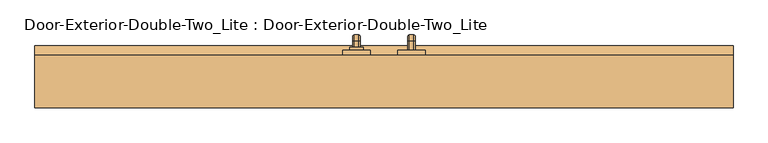
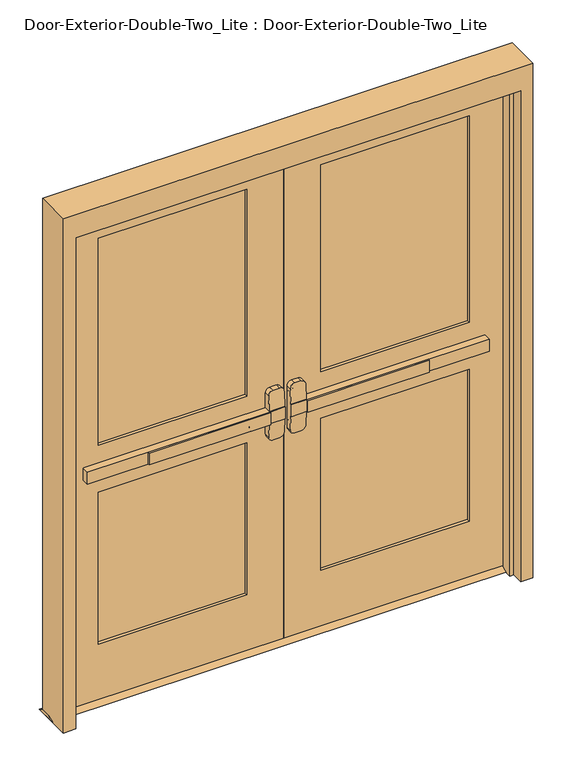
"""IFC4 building model written with IfcOpenShell, lengths in millimetres: door geometry, Door-Exterior-Double-Two_Lite : Door-Exterior-Double-Two_Lite."""

from ifc_helpers import new_model, si_unit, point, frame, frame_2d, origin, place, context, project, spatial, polyline, circle_curve, ellipse_curve, trimmed, segment, composite_curve, outline, extrude, faceted_brep, source, transform, mapped, element, save
from ifc_brep_helpers import plane_surface, cylinder_surface, revolved_surface, advanced_brep


def door_exterior_double_two_lite_door_exterior_double_two_lite_aa7d30b3(model_context):
    return source(origin(), model_context, "Body", "SolidModel", [
        extrude(outline(polyline([(-575.7333333, 48.4), (-575.7333333, 54.75), (-76.2, 54.75), (-76.2, 48.4), (-575.7333333, 48.4)])), frame((0.0, 0.0, 990.6), z_axis=(0.0, 0.0, 1.0), x_axis=(1.0, 0.0, 0.0)), (0.0, 0.0, 1.0), 50.8),
        advanced_brep(
        [(-12.7, 54.75, 1041.4), (-76.2, 54.75, 1041.4), (-825.5, 54.75, 1041.4), (-825.5, 54.75, 990.6), (-76.2, 54.75, 990.6), (-12.7, 54.75, 990.6), (-825.5, 86.5, 1041.4), (-76.2, 86.5, 1041.4), (-76.2, 86.5, 1104.9), (-57.15, 86.5, 1123.95), (-31.75, 86.5, 1123.95), (-12.7, 86.5, 1104.9), (-12.7, 86.5, 927.1), (-31.75, 86.5, 908.05), (-57.15, 86.5, 908.05), (-76.2, 86.5, 927.1), (-76.2, 86.5, 990.6), (-825.5, 86.5, 990.6), (-12.7, 57.9252467, 1041.4), (-76.2, 57.9252467, 1041.4), (-12.7, 57.9252467, 990.6), (-12.7, 62.9354269, 927.1), (-12.7, 62.9354269, 1104.9), (-76.2, 57.9252467, 990.6), (-76.2, 62.9354269, 1104.9), (-76.2, 62.9354269, 927.1), (-57.15, 64.438481, 1123.95), (-31.75, 64.438481, 1123.95), (-31.75, 64.438481, 908.05), (-57.15, 64.438481, 908.05)],
        [
            (0, 1),
            (1, 2),
            (2, 3),
            (3, 4),
            (4, 5),
            (5, 0),
            (6, 7),
            (7, 8),
            (8, 9, circle_curve(frame((-57.15, 86.5, 1104.9), z_axis=(0.0, 1.0, 0.0), x_axis=(-1.0, 0.0, 0.0)), 19.05)),
            (9, 10),
            (10, 11, circle_curve(frame((-31.75, 86.5, 1104.9), z_axis=(0.0, 1.0, 0.0), x_axis=(-1.0, 0.0, 0.0)), 19.05)),
            (11, 12),
            (12, 13, circle_curve(frame((-31.75, 86.5, 927.1), z_axis=(0.0, 1.0, 0.0), x_axis=(-1.0, 0.0, 0.0)), 19.05)),
            (13, 14),
            (14, 15, circle_curve(frame((-57.15, 86.5, 927.1), z_axis=(0.0, 1.0, 0.0), x_axis=(-1.0, 0.0, 0.0)), 19.05)),
            (15, 16),
            (16, 17),
            (17, 6),
            (0, 18),
            (18, 19),
            (19, 7),
            (6, 2),
            (5, 20),
            (20, 21),
            (21, 12),
            (11, 22),
            (22, 18),
            (16, 23),
            (23, 20),
            (3, 17),
            (19, 24),
            (24, 8),
            (15, 25),
            (25, 23),
            (9, 26),
            (26, 27),
            (27, 10),
            (13, 28),
            (28, 29),
            (29, 14),
            (29, 25, ellipse_curve(frame((-57.15, 62.9354269, 927.1), z_axis=(0.0, 0.9969018152893365, 0.07865602756830282), x_axis=(0.0, -0.07865602756830208, 0.9969018152893365)), 19.1092038, 19.05)),
            (24, 26, ellipse_curve(frame((-57.15, 62.9354269, 1104.9), z_axis=(0.0, 0.9969018152893376, -0.07865602756828934), x_axis=(0.0, -0.078656027568288, -0.9969018152893377)), 19.1092038, 19.05)),
            (27, 22, ellipse_curve(frame((-31.75, 62.9354269, 1104.9), z_axis=(0.0, 0.9969018152893376, -0.07865602756828934), x_axis=(0.0, -0.078656027568288, -0.9969018152893377)), 19.1092038, 19.05)),
            (21, 28, ellipse_curve(frame((-31.75, 62.9354269, 927.1), z_axis=(0.0, 0.9969018152893365, 0.07865602756830282), x_axis=(0.0, -0.07865602756830208, 0.9969018152893365)), 19.1092038, 19.05)),
        ],
        [
            plane_surface(frame((-12.7, 54.75, 1041.4), z_axis=(0.0, -1.0, 0.0), x_axis=(1.0, 0.0, 0.0))),
            plane_surface(frame((-12.7, 86.5, 1041.4), z_axis=(0.0, 1.0, 0.0), x_axis=(-1.0, 0.0, 0.0))),
            plane_surface(frame((-825.5, 54.75, 1041.4), z_axis=(0.0, 0.0, 1.0), x_axis=(0.0, 1.0, 0.0))),
            plane_surface(frame((-12.7, 54.75, 1041.4), z_axis=(1.0, 0.0, 0.0), x_axis=(0.0, 1.0, 0.0))),
            plane_surface(frame((-12.7, 54.75, 990.6), z_axis=(0.0, 0.0, -1.0), x_axis=(0.0, 1.0, 0.0))),
            plane_surface(frame((-825.5, 54.75, 990.6), z_axis=(-1.0, 0.0, 0.0), x_axis=(0.0, 1.0, 0.0))),
            plane_surface(frame((-76.2, 57.9252467, 927.1), z_axis=(-1.0, 0.0, 0.0), x_axis=(0.0, 1.0, 0.0))),
            plane_surface(frame((-57.15, 57.9252467, 1123.95), z_axis=(0.0, 0.0, 1.0), x_axis=(0.0, 1.0, 0.0))),
            plane_surface(frame((-31.75, 57.9252467, 908.05), z_axis=(0.0, 0.0, -1.0), x_axis=(0.0, 1.0, 0.0))),
            cylinder_surface(frame((-57.15, 86.5, 927.1), z_axis=(0.0, -1.0, 0.0), x_axis=(-1.0, 0.0, 0.0)), 19.05),
            cylinder_surface(frame((-57.15, 86.5, 1104.9), z_axis=(0.0, -1.0, 0.0), x_axis=(-1.0, 0.0, 0.0)), 19.05),
            cylinder_surface(frame((-31.75, 86.5, 1104.9), z_axis=(0.0, -1.0, 0.0), x_axis=(-1.0, 0.0, 0.0)), 19.05),
            cylinder_surface(frame((-31.75, 86.5, 927.1), z_axis=(0.0, -1.0, 0.0), x_axis=(-1.0, 0.0, 0.0)), 19.05),
            plane_surface(frame((-76.2, 57.9252467, 1041.4), z_axis=(0.0, -0.9969018152893376, 0.07865602756828934), x_axis=(1.0, 0.0, 0.0))),
            plane_surface(frame((-76.2, 64.438481, 908.05), z_axis=(0.0, -0.9969018152893365, -0.07865602756830282), x_axis=(1.0, 0.0, 0.0))),
        ],
        [
            (0, [[1, 2, 3, 4, 5, 6]]),
            (1, [[7, 8, 9, 10, 11, 12, 13, 14, 15, 16, 17, 18]]),
            (2, [[-2, -1, 19, 20, 21, -7, 22]]),
            (3, [[23, 24, 25, -12, 26, 27, -19, -6]]),
            (4, [[-17, 28, 29, -23, -5, -4, 30]]),
            (5, [[-22, -18, -30, -3]]),
            (6, [[-21, 31, 32, -8]]),
            (6, [[33, 34, -28, -16]]),
            (7, [[35, 36, 37, -10]]),
            (8, [[38, 39, 40, -14]]),
            (9, [[-40, 41, -33, -15]]),
            (10, [[-32, 42, -35, -9]]),
            (11, [[-37, 43, -26, -11]]),
            (12, [[-25, 44, -38, -13]]),
            (13, [[-27, -43, -36, -42, -31, -20]]),
            (14, [[-29, -34, -41, -39, -44, -24]]),
        ],
    ),
        extrude(outline(polyline([(130.95, 12.7), (156.35, 0.0), (61.1, 0.0), (86.5, 12.7), (130.95, 12.7)])), frame((-965.2, 0.0, 0.0), z_axis=(1.0, 0.0, 0.0), x_axis=(0.0, 1.0, 0.0)), (0.0, 0.0, 1.0), 1930.4),
        extrude(outline(polyline([(575.7333333, 48.4), (76.2, 48.4), (76.2, 54.75), (575.7333333, 54.75), (575.7333333, 48.4)])), frame((0.0, 0.0, 990.6), z_axis=(0.0, 0.0, 1.0), x_axis=(1.0, 0.0, 0.0)), (0.0, 0.0, 1.0), 50.8),
        advanced_brep(
        [(12.7, 54.75, 1041.4), (12.7, 54.75, 990.6), (76.2, 54.75, 990.6), (825.5, 54.75, 990.6), (825.5, 54.75, 1041.4), (76.2, 54.75, 1041.4), (825.5, 86.5, 1041.4), (825.5, 86.5, 990.6), (76.2, 86.5, 990.6), (76.2, 86.5, 927.1), (57.15, 86.5, 908.05), (31.75, 86.5, 908.05), (12.7, 86.5, 927.1), (12.7, 86.5, 1104.9), (31.75, 86.5, 1123.95), (57.15, 86.5, 1123.95), (76.2, 86.5, 1104.9), (76.2, 86.5, 1041.4), (76.2, 57.9252467, 1041.4), (12.7, 57.9252467, 1041.4), (12.7, 62.9354269, 1104.9), (12.7, 62.9354269, 927.1), (12.7, 57.9252467, 990.6), (76.2, 57.9252467, 990.6), (76.2, 62.9354269, 927.1), (76.2, 62.9354269, 1104.9), (31.75, 64.438481, 1123.95), (57.15, 64.438481, 1123.95), (57.15, 64.438481, 908.05), (31.75, 64.438481, 908.05)],
        [
            (0, 1),
            (1, 2),
            (2, 3),
            (3, 4),
            (4, 5),
            (5, 0),
            (6, 7),
            (7, 8),
            (8, 9),
            (9, 10, circle_curve(frame((57.15, 86.5, 927.1), z_axis=(0.0, 1.0, 0.0), x_axis=(1.0, 0.0, 0.0)), 19.05)),
            (10, 11),
            (11, 12, circle_curve(frame((31.75, 86.5, 927.1), z_axis=(0.0, 1.0, 0.0), x_axis=(1.0, 0.0, 0.0)), 19.05)),
            (12, 13),
            (13, 14, circle_curve(frame((31.75, 86.5, 1104.9), z_axis=(0.0, 1.0, 0.0), x_axis=(1.0, 0.0, 0.0)), 19.05)),
            (14, 15),
            (15, 16, circle_curve(frame((57.15, 86.5, 1104.9), z_axis=(0.0, 1.0, 0.0), x_axis=(1.0, 0.0, 0.0)), 19.05)),
            (16, 17),
            (17, 6),
            (4, 6),
            (17, 18),
            (18, 19),
            (19, 0),
            (19, 20),
            (20, 13),
            (12, 21),
            (21, 22),
            (22, 1),
            (7, 3),
            (22, 23),
            (23, 8),
            (23, 24),
            (24, 9),
            (16, 25),
            (25, 18),
            (14, 26),
            (26, 27),
            (27, 15),
            (10, 28),
            (28, 29),
            (29, 11),
            (24, 28, ellipse_curve(frame((57.15, 62.9354269, 927.1), z_axis=(0.0, 0.9969018152893365, 0.07865602756830282), x_axis=(0.0, -0.07865602756830208, 0.9969018152893365)), 19.1092038, 19.05)),
            (27, 25, ellipse_curve(frame((57.15, 62.9354269, 1104.9), z_axis=(0.0, 0.9969018152893376, -0.07865602756828934), x_axis=(0.0, -0.078656027568288, -0.9969018152893377)), 19.1092038, 19.05)),
            (20, 26, ellipse_curve(frame((31.75, 62.9354269, 1104.9), z_axis=(0.0, 0.9969018152893376, -0.07865602756828934), x_axis=(0.0, -0.078656027568288, -0.9969018152893377)), 19.1092038, 19.05)),
            (29, 21, ellipse_curve(frame((31.75, 62.9354269, 927.1), z_axis=(0.0, 0.9969018152893365, 0.07865602756830282), x_axis=(0.0, -0.07865602756830208, 0.9969018152893365)), 19.1092038, 19.05)),
        ],
        [
            plane_surface(frame((12.7, 54.75, 1041.4), z_axis=(0.0, -1.0, 0.0), x_axis=(-1.0, 0.0, 0.0))),
            plane_surface(frame((12.7, 86.5, 1041.4), z_axis=(0.0, 1.0, 0.0), x_axis=(1.0, 0.0, 0.0))),
            plane_surface(frame((825.5, 54.75, 1041.4), z_axis=(0.0, 0.0, 1.0), x_axis=(0.0, 1.0, 0.0))),
            plane_surface(frame((12.7, 54.75, 1041.4), z_axis=(-1.0, 0.0, 0.0), x_axis=(0.0, 1.0, 0.0))),
            plane_surface(frame((12.7, 54.75, 990.6), z_axis=(0.0, 0.0, -1.0), x_axis=(0.0, 1.0, 0.0))),
            plane_surface(frame((825.5, 54.75, 990.6), z_axis=(1.0, 0.0, 0.0), x_axis=(0.0, 1.0, 0.0))),
            plane_surface(frame((76.2, 57.9252467, 927.1), z_axis=(1.0, 0.0, 0.0), x_axis=(0.0, 1.0, 0.0))),
            plane_surface(frame((57.15, 57.9252467, 1123.95), z_axis=(0.0, 0.0, 1.0), x_axis=(0.0, 1.0, 0.0))),
            plane_surface(frame((31.75, 57.9252467, 908.05), z_axis=(0.0, 0.0, -1.0), x_axis=(0.0, 1.0, 0.0))),
            cylinder_surface(frame((57.15, 86.5, 927.1), z_axis=(0.0, -1.0, 0.0), x_axis=(1.0, 0.0, 0.0)), 19.05),
            cylinder_surface(frame((57.15, 86.5, 1104.9), z_axis=(0.0, -1.0, 0.0), x_axis=(1.0, 0.0, 0.0)), 19.05),
            cylinder_surface(frame((31.75, 86.5, 1104.9), z_axis=(0.0, -1.0, 0.0), x_axis=(1.0, 0.0, 0.0)), 19.05),
            cylinder_surface(frame((31.75, 86.5, 927.1), z_axis=(0.0, -1.0, 0.0), x_axis=(1.0, 0.0, 0.0)), 19.05),
            plane_surface(frame((76.2, 57.9252467, 1041.4), z_axis=(0.0, -0.9969018152893376, 0.07865602756828934), x_axis=(-1.0, 0.0, 0.0))),
            plane_surface(frame((76.2, 64.438481, 908.05), z_axis=(0.0, -0.9969018152893365, -0.07865602756830282), x_axis=(-1.0, 0.0, 0.0))),
        ],
        [
            (0, [[1, 2, 3, 4, 5, 6]]),
            (1, [[7, 8, 9, 10, 11, 12, 13, 14, 15, 16, 17, 18]]),
            (2, [[19, -18, 20, 21, 22, -6, -5]]),
            (3, [[-1, -22, 23, 24, -13, 25, 26, 27]]),
            (4, [[28, -3, -2, -27, 29, 30, -8]]),
            (5, [[-4, -28, -7, -19]]),
            (6, [[-9, -30, 31, 32]]),
            (6, [[-17, 33, 34, -20]]),
            (7, [[-15, 35, 36, 37]]),
            (8, [[-11, 38, 39, 40]]),
            (9, [[-10, -32, 41, -38]]),
            (10, [[-16, -37, 42, -33]]),
            (11, [[-14, -24, 43, -35]]),
            (12, [[-12, -40, 44, -25]]),
            (13, [[-21, -34, -42, -36, -43, -23]]),
            (14, [[-26, -44, -39, -41, -31, -29]]),
        ],
    ),
        advanced_brep(
        [(66.2, 143.65, 1017.190625), (66.2, 143.65, 1014.809375), (69.771875, 143.65, 1011.2375), (82.6284594, 143.65, 1011.2375), (86.2, 143.65, 1014.8090406), (86.2, 143.65, 1017.190625), (82.628125, 143.65, 1020.7625), (69.771875, 143.65, 1020.7625), (66.2, 143.65, 887.809375), (69.771875, 143.65, 884.2375), (82.628125, 143.65, 884.2375), (86.2, 143.65, 887.809375), (86.2, 143.65, 890.1909594), (82.6284594, 143.65, 893.7625), (69.771875, 143.65, 893.7625), (66.2, 143.65, 890.190625), (66.2, 169.05, 1017.190625), (66.2, 182.940625, 1003.3), (66.2, 182.940625, 901.7), (66.2, 169.05, 887.809375), (66.2, 169.05, 890.190625), (66.2, 180.559375, 901.7), (66.2, 180.559375, 1003.3), (66.2, 169.05, 1014.809375), (69.771875, 169.05, 1011.2375), (82.6284594, 169.05, 1011.2375), (86.2, 169.05, 1014.8090406), (86.2, 180.5590406, 1003.3), (86.2, 180.5590406, 901.7), (86.2, 169.05, 890.1909594), (86.2, 169.05, 887.809375), (86.2, 182.940625, 901.7), (86.2, 182.940625, 1003.3), (86.2, 169.05, 1017.190625), (82.628125, 169.05, 1020.7625), (69.771875, 169.05, 1020.7625), (69.771875, 176.9875, 1003.3), (82.6284594, 176.9875, 1003.3), (82.628125, 186.5125, 1003.3), (69.771875, 186.5125, 1003.3), (69.771875, 176.9875, 901.7), (82.6284594, 176.9875, 901.7), (82.628125, 186.5125, 901.7), (69.771875, 186.5125, 901.7), (69.771875, 169.05, 893.7625), (82.6284594, 169.05, 893.7625), (82.628125, 169.05, 884.2375), (69.771875, 169.05, 884.2375)],
        [
            (0, 1),
            (1, 2, circle_curve(frame((69.771875, 143.65, 1014.809375), z_axis=(0.0, -1.0, 0.0), x_axis=(0.0, 0.0, 1.0)), 3.571875)),
            (2, 3),
            (3, 4, circle_curve(frame((82.6284594, 143.65, 1014.8090406), z_axis=(0.0, -1.0, 0.0), x_axis=(0.0, 0.0, 1.0)), 3.5715406)),
            (4, 5),
            (5, 6, circle_curve(frame((82.628125, 143.65, 1017.190625), z_axis=(0.0, -1.0, 0.0), x_axis=(0.0, 0.0, 1.0)), 3.571875)),
            (6, 7),
            (7, 0, circle_curve(frame((69.771875, 143.65, 1017.190625), z_axis=(0.0, -1.0, 0.0), x_axis=(0.0, 0.0, 1.0)), 3.571875)),
            (8, 9, circle_curve(frame((69.771875, 143.65, 887.809375), z_axis=(0.0, -1.0, 0.0), x_axis=(0.0, 0.0, -1.0)), 3.571875)),
            (9, 10),
            (10, 11, circle_curve(frame((82.628125, 143.65, 887.809375), z_axis=(0.0, -1.0, 0.0), x_axis=(0.0, 0.0, -1.0)), 3.571875)),
            (11, 12),
            (12, 13, circle_curve(frame((82.6284594, 143.65, 890.1909594), z_axis=(0.0, -1.0, 0.0), x_axis=(0.0, 0.0, -1.0)), 3.5715406)),
            (13, 14),
            (14, 15, circle_curve(frame((69.771875, 143.65, 890.190625), z_axis=(0.0, -1.0, 0.0), x_axis=(0.0, 0.0, -1.0)), 3.571875)),
            (15, 8),
            (0, 16),
            (16, 17, circle_curve(frame((66.2, 169.05, 1003.3), z_axis=(-1.0, 0.0, 0.0), x_axis=(0.0, 0.0, 1.0)), 13.890625)),
            (17, 18),
            (18, 19, circle_curve(frame((66.2, 169.05, 901.7), z_axis=(-1.0, 0.0, 0.0), x_axis=(0.0, 1.0, 0.0)), 13.890625)),
            (19, 8),
            (15, 20),
            (20, 21, circle_curve(frame((66.2, 169.05, 901.7), z_axis=(1.0, 0.0, 0.0), x_axis=(0.0, 1.0, 0.0)), 11.509375)),
            (21, 22),
            (22, 23, circle_curve(frame((66.2, 169.05, 1003.3), z_axis=(1.0, 0.0, 0.0), x_axis=(0.0, 0.0, 1.0)), 11.509375)),
            (23, 1),
            (23, 24, circle_curve(frame((69.771875, 169.05, 1014.809375), z_axis=(0.0, -1.0, 0.0), x_axis=(0.0, 0.0, 1.0)), 3.571875)),
            (24, 2),
            (24, 25),
            (25, 3),
            (25, 26, circle_curve(frame((82.6284594, 169.05, 1014.8090406), z_axis=(0.0, -1.0, 0.0), x_axis=(0.0, 0.0, 1.0)), 3.5715406)),
            (26, 4),
            (26, 27, circle_curve(frame((86.2, 169.05, 1003.3), z_axis=(-1.0, 0.0, 0.0), x_axis=(0.0, 0.0, 1.0)), 11.5090406)),
            (27, 28),
            (28, 29, circle_curve(frame((86.2, 169.05, 901.7), z_axis=(-1.0, 0.0, 0.0), x_axis=(0.0, 1.0, 0.0)), 11.5090406)),
            (29, 12),
            (11, 30),
            (30, 31, circle_curve(frame((86.2, 169.05, 901.7), z_axis=(1.0, 0.0, 0.0), x_axis=(0.0, 1.0, 0.0)), 13.890625)),
            (31, 32),
            (32, 33, circle_curve(frame((86.2, 169.05, 1003.3), z_axis=(1.0, 0.0, 0.0), x_axis=(0.0, 0.0, 1.0)), 13.890625)),
            (33, 5),
            (33, 34, circle_curve(frame((82.628125, 169.05, 1017.190625), z_axis=(0.0, -1.0, 0.0), x_axis=(0.0, 0.0, 1.0)), 3.571875)),
            (34, 6),
            (34, 35),
            (35, 7),
            (35, 16, circle_curve(frame((69.771875, 169.05, 1017.190625), z_axis=(0.0, -1.0, 0.0), x_axis=(0.0, 0.0, 1.0)), 3.571875)),
            (36, 24, circle_curve(frame((69.771875, 169.05, 1003.3), z_axis=(1.0, 0.0, 0.0), x_axis=(0.0, 0.0, 1.0)), 7.9375)),
            (22, 36, circle_curve(frame((69.771875, 180.559375, 1003.3), z_axis=(0.0, 0.0, 1.0), x_axis=(0.0, 1.0, 0.0)), 3.571875)),
            (37, 25, circle_curve(frame((82.6284594, 169.05, 1003.3), z_axis=(1.0, 0.0, 0.0), x_axis=(0.0, 0.0, 1.0)), 7.9375)),
            (36, 37),
            (37, 27, circle_curve(frame((82.6284594, 180.5590406, 1003.3), z_axis=(0.0, 0.0, 1.0), x_axis=(0.0, 1.0, 0.0)), 3.5715406)),
            (38, 34, circle_curve(frame((82.628125, 169.05, 1003.3), z_axis=(1.0, 0.0, 0.0), x_axis=(0.0, 0.0, 1.0)), 17.4625)),
            (32, 38, circle_curve(frame((82.628125, 182.940625, 1003.3), z_axis=(0.0, 0.0, 1.0), x_axis=(0.0, 1.0, 0.0)), 3.571875)),
            (39, 35, circle_curve(frame((69.771875, 169.05, 1003.3), z_axis=(1.0, 0.0, 0.0), x_axis=(0.0, 0.0, 1.0)), 17.4625)),
            (38, 39),
            (39, 17, circle_curve(frame((69.771875, 182.940625, 1003.3), z_axis=(0.0, 0.0, 1.0), x_axis=(0.0, 1.0, 0.0)), 3.571875)),
            (21, 40, circle_curve(frame((69.771875, 180.559375, 901.7), z_axis=(0.0, 0.0, 1.0), x_axis=(0.0, 1.0, 0.0)), 3.571875)),
            (40, 36),
            (40, 41),
            (41, 37),
            (41, 28, circle_curve(frame((82.6284594, 180.5590406, 901.7), z_axis=(0.0, 0.0, 1.0), x_axis=(0.0, 1.0, 0.0)), 3.5715406)),
            (31, 42, circle_curve(frame((82.628125, 182.940625, 901.7), z_axis=(0.0, 0.0, 1.0), x_axis=(0.0, 1.0, 0.0)), 3.571875)),
            (42, 38),
            (42, 43),
            (43, 39),
            (43, 18, circle_curve(frame((69.771875, 182.940625, 901.7), z_axis=(0.0, 0.0, 1.0), x_axis=(0.0, 1.0, 0.0)), 3.571875)),
            (44, 40, circle_curve(frame((69.771875, 169.05, 901.7), z_axis=(1.0, 0.0, 0.0), x_axis=(0.0, 1.0, 0.0)), 7.9375)),
            (20, 44, circle_curve(frame((69.771875, 169.05, 890.190625), z_axis=(0.0, 1.0, 0.0), x_axis=(0.0, 0.0, -1.0)), 3.571875)),
            (45, 41, circle_curve(frame((82.6284594, 169.05, 901.7), z_axis=(1.0, 0.0, 0.0), x_axis=(0.0, 1.0, 0.0)), 7.9375)),
            (44, 45),
            (45, 29, circle_curve(frame((82.6284594, 169.05, 890.1909594), z_axis=(0.0, 1.0, 0.0), x_axis=(0.0, 0.0, -1.0)), 3.5715406)),
            (46, 42, circle_curve(frame((82.628125, 169.05, 901.7), z_axis=(1.0, 0.0, 0.0), x_axis=(0.0, 1.0, 0.0)), 17.4625)),
            (30, 46, circle_curve(frame((82.628125, 169.05, 887.809375), z_axis=(0.0, 1.0, 0.0), x_axis=(0.0, 0.0, -1.0)), 3.571875)),
            (47, 43, circle_curve(frame((69.771875, 169.05, 901.7), z_axis=(1.0, 0.0, 0.0), x_axis=(0.0, 1.0, 0.0)), 17.4625)),
            (46, 47),
            (47, 19, circle_curve(frame((69.771875, 169.05, 887.809375), z_axis=(0.0, 1.0, 0.0), x_axis=(0.0, 0.0, -1.0)), 3.571875)),
            (14, 44),
            (13, 45),
            (10, 46),
            (9, 47),
        ],
        [
            plane_surface(frame((76.2, 143.65, 1016.0), z_axis=(0.0, -1.0, 0.0), x_axis=(1.0, 0.0, 0.0))),
            plane_surface(frame((76.2, 143.65, 889.0), z_axis=(0.0, -1.0, 0.0), x_axis=(1.0, 0.0, 0.0))),
            plane_surface(frame((66.2, 143.65, 1017.190625), z_axis=(-1.0, 0.0, 0.0), x_axis=(0.0, 1.0, 0.0))),
            cylinder_surface(frame((69.771875, 143.65, 1014.809375), z_axis=(0.0, -1.0, 0.0), x_axis=(0.0, 0.0, 1.0)), 3.571875),
            plane_surface(frame((69.771875, 143.65, 1011.2375), z_axis=(0.0, 0.0, -1.0), x_axis=(0.0, 1.0, 0.0))),
            cylinder_surface(frame((82.6284594, 143.65, 1014.8090406), z_axis=(0.0, -1.0, 0.0), x_axis=(0.0, 0.0, 1.0)), 3.5715406),
            plane_surface(frame((86.2, 143.65, 1014.8090406), z_axis=(1.0, 0.0, 0.0), x_axis=(0.0, 1.0, 0.0))),
            cylinder_surface(frame((82.628125, 143.65, 1017.190625), z_axis=(0.0, -1.0, 0.0), x_axis=(0.0, 0.0, 1.0)), 3.571875),
            plane_surface(frame((82.628125, 143.65, 1020.7625), z_axis=(0.0, 0.0, 1.0), x_axis=(0.0, 1.0, 0.0))),
            cylinder_surface(frame((69.771875, 143.65, 1017.190625), z_axis=(0.0, -1.0, 0.0), x_axis=(0.0, 0.0, 1.0)), 3.571875),
            revolved_surface(trimmed(ellipse_curve(frame((69.771875, 169.05, 1014.809375), z_axis=(0.0, -1.0, 0.0), x_axis=(0.0, 0.0, 1.0)), 3.571875, 3.571875), [point((66.2, 169.05, 1014.809375))], [point((69.771875, 169.05, 1011.2375))], True, "CARTESIAN"), (76.2, 169.05, 1003.3), (-1.0, 0.0, 0.0)),
            revolved_surface(polyline([(69.771875, 169.05, 1011.2375), (82.6284594, 169.05, 1011.2375)]), (76.2, 169.05, 1003.3), (-1.0, 0.0, 0.0)),
            revolved_surface(trimmed(ellipse_curve(frame((82.6284594, 169.05, 1014.8090406), z_axis=(0.0, -1.0, 0.0), x_axis=(0.0, 0.0, 1.0)), 3.5715406, 3.5715406), [point((82.6284594, 169.05, 1011.2375))], [point((86.2, 169.05, 1014.8090406))], True, "CARTESIAN"), (76.2, 169.05, 1003.3), (-1.0, 0.0, 0.0)),
            revolved_surface(trimmed(ellipse_curve(frame((82.628125, 169.05, 1017.190625), z_axis=(0.0, -1.0, 0.0), x_axis=(0.0, 0.0, 1.0)), 3.571875, 3.571875), [point((86.2, 169.05, 1017.190625))], [point((82.628125, 169.05, 1020.7625))], True, "CARTESIAN"), (76.2, 169.05, 1003.3), (-1.0, 0.0, 0.0)),
            cylinder_surface(frame((76.2, 169.05, 1003.3), z_axis=(-1.0, 0.0, 0.0), x_axis=(0.0, 0.0, 1.0)), 17.4625),
            revolved_surface(trimmed(ellipse_curve(frame((69.771875, 169.05, 1017.190625), z_axis=(0.0, -1.0, 0.0), x_axis=(0.0, 0.0, 1.0)), 3.571875, 3.571875), [point((69.771875, 169.05, 1020.7625))], [point((66.2, 169.05, 1017.190625))], True, "CARTESIAN"), (76.2, 169.05, 1003.3), (-1.0, 0.0, 0.0)),
            cylinder_surface(frame((69.771875, 180.559375, 1003.3), z_axis=(0.0, 0.0, 1.0), x_axis=(0.0, 1.0, 0.0)), 3.571875),
            plane_surface(frame((69.771875, 176.9875, 1003.3), z_axis=(0.0, -1.0, 0.0), x_axis=(0.0, 0.0, -1.0))),
            cylinder_surface(frame((82.6284594, 180.5590406, 1003.3), z_axis=(0.0, 0.0, 1.0), x_axis=(0.0, 1.0, 0.0)), 3.5715406),
            cylinder_surface(frame((82.628125, 182.940625, 1003.3), z_axis=(0.0, 0.0, 1.0), x_axis=(0.0, 1.0, 0.0)), 3.571875),
            plane_surface(frame((82.628125, 186.5125, 1003.3), z_axis=(0.0, 1.0, 0.0), x_axis=(0.0, 0.0, -1.0))),
            cylinder_surface(frame((69.771875, 182.940625, 1003.3), z_axis=(0.0, 0.0, 1.0), x_axis=(0.0, 1.0, 0.0)), 3.571875),
            revolved_surface(trimmed(ellipse_curve(frame((69.771875, 180.559375, 901.7), z_axis=(0.0, 0.0, 1.0), x_axis=(0.0, 1.0, 0.0)), 3.571875, 3.571875), [point((66.2, 180.559375, 901.7))], [point((69.771875, 176.9875, 901.7))], True, "CARTESIAN"), (76.2, 169.05, 901.7), (-1.0, 0.0, 0.0)),
            revolved_surface(polyline([(69.771875, 176.9875, 901.7), (82.6284594, 176.9875, 901.7)]), (76.2, 169.05, 901.7), (-1.0, 0.0, 0.0)),
            revolved_surface(trimmed(ellipse_curve(frame((82.6284594, 180.5590406, 901.7), z_axis=(0.0, 0.0, 1.0), x_axis=(0.0, 1.0, 0.0)), 3.5715406, 3.5715406), [point((82.6284594, 176.9875, 901.7))], [point((86.2, 180.5590406, 901.7))], True, "CARTESIAN"), (76.2, 169.05, 901.7), (-1.0, 0.0, 0.0)),
            revolved_surface(trimmed(ellipse_curve(frame((82.628125, 182.940625, 901.7), z_axis=(0.0, 0.0, 1.0), x_axis=(0.0, 1.0, 0.0)), 3.571875, 3.571875), [point((86.2, 182.940625, 901.7))], [point((82.628125, 186.5125, 901.7))], True, "CARTESIAN"), (76.2, 169.05, 901.7), (-1.0, 0.0, 0.0)),
            cylinder_surface(frame((76.2, 169.05, 901.7), z_axis=(-1.0, 0.0, 0.0), x_axis=(0.0, 1.0, 0.0)), 17.4625),
            revolved_surface(trimmed(ellipse_curve(frame((69.771875, 182.940625, 901.7), z_axis=(0.0, 0.0, 1.0), x_axis=(0.0, 1.0, 0.0)), 3.571875, 3.571875), [point((69.771875, 186.5125, 901.7))], [point((66.2, 182.940625, 901.7))], True, "CARTESIAN"), (76.2, 169.05, 901.7), (-1.0, 0.0, 0.0)),
            cylinder_surface(frame((69.771875, 169.05, 890.190625), z_axis=(0.0, 1.0, 0.0), x_axis=(0.0, 0.0, -1.0)), 3.571875),
            plane_surface(frame((69.771875, 169.05, 893.7625), z_axis=(0.0, 0.0, 1.0), x_axis=(0.0, -1.0, 0.0))),
            cylinder_surface(frame((82.6284594, 169.05, 890.1909594), z_axis=(0.0, 1.0, 0.0), x_axis=(0.0, 0.0, -1.0)), 3.5715406),
            cylinder_surface(frame((82.628125, 169.05, 887.809375), z_axis=(0.0, 1.0, 0.0), x_axis=(0.0, 0.0, -1.0)), 3.571875),
            plane_surface(frame((82.628125, 169.05, 884.2375), z_axis=(0.0, 0.0, -1.0), x_axis=(0.0, -1.0, 0.0))),
            cylinder_surface(frame((69.771875, 169.05, 887.809375), z_axis=(0.0, 1.0, 0.0), x_axis=(0.0, 0.0, -1.0)), 3.571875),
        ],
        [
            (0, [[1, 2, 3, 4, 5, 6, 7, 8]]),
            (1, [[9, 10, 11, 12, 13, 14, 15, 16]]),
            (2, [[-1, 17, 18, 19, 20, 21, -16, 22, 23, 24, 25, 26]]),
            (3, [[-2, -26, 27, 28]]),
            (4, [[-3, -28, 29, 30]]),
            (5, [[-4, -30, 31, 32]]),
            (6, [[-5, -32, 33, 34, 35, 36, -12, 37, 38, 39, 40, 41]]),
            (7, [[-6, -41, 42, 43]]),
            (8, [[-7, -43, 44, 45]]),
            (9, [[-8, -45, 46, -17]]),
            (10, [[47, -27, -25, 48]]),
            (11, [[49, -29, -47, 50]]),
            (12, [[-33, -31, -49, 51]]),
            (13, [[52, -42, -40, 53]]),
            (14, [[54, -44, -52, 55]]),
            (15, [[-18, -46, -54, 56]]),
            (16, [[-48, -24, 57, 58]]),
            (17, [[-50, -58, 59, 60]]),
            (18, [[-51, -60, 61, -34]]),
            (19, [[-53, -39, 62, 63]]),
            (20, [[-55, -63, 64, 65]]),
            (21, [[-56, -65, 66, -19]]),
            (22, [[67, -57, -23, 68]]),
            (23, [[69, -59, -67, 70]]),
            (24, [[-35, -61, -69, 71]]),
            (25, [[72, -62, -38, 73]]),
            (26, [[74, -64, -72, 75]]),
            (27, [[-20, -66, -74, 76]]),
            (28, [[-68, -22, -15, 77]]),
            (29, [[-70, -77, -14, 78]]),
            (30, [[-71, -78, -13, -36]]),
            (31, [[-73, -37, -11, 79]]),
            (32, [[-75, -79, -10, 80]]),
            (33, [[-76, -80, -9, -21]]),
        ],
    ),
        extrude(outline(composite_curve([segment(trimmed(circle_curve(frame_2d((1113.0338574, 76.2)), 89.3016225), [point((1193.8, 114.3))], [point((1193.8, 38.1))], False, "CARTESIAN"), True, "CONTINUOUS"), segment(polyline([(1193.8, 38.1), (838.2, 38.1)]), True, "CONTINUOUS"), segment(trimmed(circle_curve(frame_2d((918.9661426, 76.2)), 89.3016225), [point((838.2, 38.1))], [point((838.2, 114.3))], False, "CARTESIAN"), True, "CONTINUOUS"), segment(polyline([(838.2, 114.3), (1193.8, 114.3)]), True, "CONTINUOUS")], self_intersect=False)), frame((0.0, 130.95, 0.0), z_axis=(0.0, 1.0, 0.0), x_axis=(0.0, 0.0, 1.0)), (0.0, 0.0, 1.0), 12.7),
        advanced_brep(
        [(-86.2, 143.65, 1017.190625), (-86.2, 143.65, 1014.809375), (-82.628125, 143.65, 1011.2375), (-69.7715406, 143.65, 1011.2375), (-66.2, 143.65, 1014.8090406), (-66.2, 143.65, 1017.190625), (-69.771875, 143.65, 1020.7625), (-82.628125, 143.65, 1020.7625), (-86.2, 143.65, 887.809375), (-82.628125, 143.65, 884.2375), (-69.771875, 143.65, 884.2375), (-66.2, 143.65, 887.809375), (-66.2, 143.65, 890.1909594), (-69.7715406, 143.65, 893.7625), (-82.628125, 143.65, 893.7625), (-86.2, 143.65, 890.190625), (-86.2, 169.05, 1017.190625), (-86.2, 182.940625, 1003.3), (-86.2, 182.940625, 901.7), (-86.2, 169.05, 887.809375), (-86.2, 169.05, 890.190625), (-86.2, 180.559375, 901.7), (-86.2, 180.559375, 1003.3), (-86.2, 169.05, 1014.809375), (-82.628125, 169.05, 1011.2375), (-69.7715406, 169.05, 1011.2375), (-66.2, 169.05, 1014.8090406), (-66.2, 180.5590406, 1003.3), (-66.2, 180.5590406, 901.7), (-66.2, 169.05, 890.1909594), (-66.2, 169.05, 887.809375), (-66.2, 182.940625, 901.7), (-66.2, 182.940625, 1003.3), (-66.2, 169.05, 1017.190625), (-69.771875, 169.05, 1020.7625), (-82.628125, 169.05, 1020.7625), (-82.628125, 176.9875, 1003.3), (-69.7715406, 176.9875, 1003.3), (-69.771875, 186.5125, 1003.3), (-82.628125, 186.5125, 1003.3), (-82.628125, 176.9875, 901.7), (-69.7715406, 176.9875, 901.7), (-69.771875, 186.5125, 901.7), (-82.628125, 186.5125, 901.7), (-82.628125, 169.05, 893.7625), (-69.7715406, 169.05, 893.7625), (-69.771875, 169.05, 884.2375), (-82.628125, 169.05, 884.2375)],
        [
            (0, 1),
            (1, 2, circle_curve(frame((-82.628125, 143.65, 1014.809375), z_axis=(0.0, -1.0, 0.0), x_axis=(0.0, 0.0, 1.0)), 3.571875)),
            (2, 3),
            (3, 4, circle_curve(frame((-69.7715406, 143.65, 1014.8090406), z_axis=(0.0, -1.0, 0.0), x_axis=(0.0, 0.0, 1.0)), 3.5715406)),
            (4, 5),
            (5, 6, circle_curve(frame((-69.771875, 143.65, 1017.190625), z_axis=(0.0, -1.0, 0.0), x_axis=(0.0, 0.0, 1.0)), 3.571875)),
            (6, 7),
            (7, 0, circle_curve(frame((-82.628125, 143.65, 1017.190625), z_axis=(0.0, -1.0, 0.0), x_axis=(0.0, 0.0, 1.0)), 3.571875)),
            (8, 9, circle_curve(frame((-82.628125, 143.65, 887.809375), z_axis=(0.0, -1.0, 0.0), x_axis=(0.0, 0.0, -1.0)), 3.571875)),
            (9, 10),
            (10, 11, circle_curve(frame((-69.771875, 143.65, 887.809375), z_axis=(0.0, -1.0, 0.0), x_axis=(0.0, 0.0, -1.0)), 3.571875)),
            (11, 12),
            (12, 13, circle_curve(frame((-69.7715406, 143.65, 890.1909594), z_axis=(0.0, -1.0, 0.0), x_axis=(0.0, 0.0, -1.0)), 3.5715406)),
            (13, 14),
            (14, 15, circle_curve(frame((-82.628125, 143.65, 890.190625), z_axis=(0.0, -1.0, 0.0), x_axis=(0.0, 0.0, -1.0)), 3.571875)),
            (15, 8),
            (0, 16),
            (16, 17, circle_curve(frame((-86.2, 169.05, 1003.3), z_axis=(-1.0, 0.0, 0.0), x_axis=(0.0, 0.0, 1.0)), 13.890625)),
            (17, 18),
            (18, 19, circle_curve(frame((-86.2, 169.05, 901.7), z_axis=(-1.0, 0.0, 0.0), x_axis=(0.0, 1.0, 0.0)), 13.890625)),
            (19, 8),
            (15, 20),
            (20, 21, circle_curve(frame((-86.2, 169.05, 901.7), z_axis=(1.0, 0.0, 0.0), x_axis=(0.0, 1.0, 0.0)), 11.509375)),
            (21, 22),
            (22, 23, circle_curve(frame((-86.2, 169.05, 1003.3), z_axis=(1.0, 0.0, 0.0), x_axis=(0.0, 0.0, 1.0)), 11.509375)),
            (23, 1),
            (23, 24, circle_curve(frame((-82.628125, 169.05, 1014.809375), z_axis=(0.0, -1.0, 0.0), x_axis=(0.0, 0.0, 1.0)), 3.571875)),
            (24, 2),
            (24, 25),
            (25, 3),
            (25, 26, circle_curve(frame((-69.7715406, 169.05, 1014.8090406), z_axis=(0.0, -1.0, 0.0), x_axis=(0.0, 0.0, 1.0)), 3.5715406)),
            (26, 4),
            (26, 27, circle_curve(frame((-66.2, 169.05, 1003.3), z_axis=(-1.0, 0.0, 0.0), x_axis=(0.0, 0.0, 1.0)), 11.5090406)),
            (27, 28),
            (28, 29, circle_curve(frame((-66.2, 169.05, 901.7), z_axis=(-1.0, 0.0, 0.0), x_axis=(0.0, 1.0, 0.0)), 11.5090406)),
            (29, 12),
            (11, 30),
            (30, 31, circle_curve(frame((-66.2, 169.05, 901.7), z_axis=(1.0, 0.0, 0.0), x_axis=(0.0, 1.0, 0.0)), 13.890625)),
            (31, 32),
            (32, 33, circle_curve(frame((-66.2, 169.05, 1003.3), z_axis=(1.0, 0.0, 0.0), x_axis=(0.0, 0.0, 1.0)), 13.890625)),
            (33, 5),
            (33, 34, circle_curve(frame((-69.771875, 169.05, 1017.190625), z_axis=(0.0, -1.0, 0.0), x_axis=(0.0, 0.0, 1.0)), 3.571875)),
            (34, 6),
            (34, 35),
            (35, 7),
            (35, 16, circle_curve(frame((-82.628125, 169.05, 1017.190625), z_axis=(0.0, -1.0, 0.0), x_axis=(0.0, 0.0, 1.0)), 3.571875)),
            (36, 24, circle_curve(frame((-82.628125, 169.05, 1003.3), z_axis=(1.0, 0.0, 0.0), x_axis=(0.0, 0.0, 1.0)), 7.9375)),
            (22, 36, circle_curve(frame((-82.628125, 180.559375, 1003.3), z_axis=(0.0, 0.0, 1.0), x_axis=(0.0, 1.0, 0.0)), 3.571875)),
            (37, 25, circle_curve(frame((-69.7715406, 169.05, 1003.3), z_axis=(1.0, 0.0, 0.0), x_axis=(0.0, 0.0, 1.0)), 7.9375)),
            (36, 37),
            (37, 27, circle_curve(frame((-69.7715406, 180.5590406, 1003.3), z_axis=(0.0, 0.0, 1.0), x_axis=(0.0, 1.0, 0.0)), 3.5715406)),
            (38, 34, circle_curve(frame((-69.771875, 169.05, 1003.3), z_axis=(1.0, 0.0, 0.0), x_axis=(0.0, 0.0, 1.0)), 17.4625)),
            (32, 38, circle_curve(frame((-69.771875, 182.940625, 1003.3), z_axis=(0.0, 0.0, 1.0), x_axis=(0.0, 1.0, 0.0)), 3.571875)),
            (39, 35, circle_curve(frame((-82.628125, 169.05, 1003.3), z_axis=(1.0, 0.0, 0.0), x_axis=(0.0, 0.0, 1.0)), 17.4625)),
            (38, 39),
            (39, 17, circle_curve(frame((-82.628125, 182.940625, 1003.3), z_axis=(0.0, 0.0, 1.0), x_axis=(0.0, 1.0, 0.0)), 3.571875)),
            (21, 40, circle_curve(frame((-82.628125, 180.559375, 901.7), z_axis=(0.0, 0.0, 1.0), x_axis=(0.0, 1.0, 0.0)), 3.571875)),
            (40, 36),
            (40, 41),
            (41, 37),
            (41, 28, circle_curve(frame((-69.7715406, 180.5590406, 901.7), z_axis=(0.0, 0.0, 1.0), x_axis=(0.0, 1.0, 0.0)), 3.5715406)),
            (31, 42, circle_curve(frame((-69.771875, 182.940625, 901.7), z_axis=(0.0, 0.0, 1.0), x_axis=(0.0, 1.0, 0.0)), 3.571875)),
            (42, 38),
            (42, 43),
            (43, 39),
            (43, 18, circle_curve(frame((-82.628125, 182.940625, 901.7), z_axis=(0.0, 0.0, 1.0), x_axis=(0.0, 1.0, 0.0)), 3.571875)),
            (44, 40, circle_curve(frame((-82.628125, 169.05, 901.7), z_axis=(1.0, 0.0, 0.0), x_axis=(0.0, 1.0, 0.0)), 7.9375)),
            (20, 44, circle_curve(frame((-82.628125, 169.05, 890.190625), z_axis=(0.0, 1.0, 0.0), x_axis=(0.0, 0.0, -1.0)), 3.571875)),
            (45, 41, circle_curve(frame((-69.7715406, 169.05, 901.7), z_axis=(1.0, 0.0, 0.0), x_axis=(0.0, 1.0, 0.0)), 7.9375)),
            (44, 45),
            (45, 29, circle_curve(frame((-69.7715406, 169.05, 890.1909594), z_axis=(0.0, 1.0, 0.0), x_axis=(0.0, 0.0, -1.0)), 3.5715406)),
            (46, 42, circle_curve(frame((-69.771875, 169.05, 901.7), z_axis=(1.0, 0.0, 0.0), x_axis=(0.0, 1.0, 0.0)), 17.4625)),
            (30, 46, circle_curve(frame((-69.771875, 169.05, 887.809375), z_axis=(0.0, 1.0, 0.0), x_axis=(0.0, 0.0, -1.0)), 3.571875)),
            (47, 43, circle_curve(frame((-82.628125, 169.05, 901.7), z_axis=(1.0, 0.0, 0.0), x_axis=(0.0, 1.0, 0.0)), 17.4625)),
            (46, 47),
            (47, 19, circle_curve(frame((-82.628125, 169.05, 887.809375), z_axis=(0.0, 1.0, 0.0), x_axis=(0.0, 0.0, -1.0)), 3.571875)),
            (14, 44),
            (13, 45),
            (10, 46),
            (9, 47),
        ],
        [
            plane_surface(frame((-76.2, 143.65, 1016.0), z_axis=(0.0, -1.0, 0.0), x_axis=(1.0, 0.0, 0.0))),
            plane_surface(frame((-76.2, 143.65, 889.0), z_axis=(0.0, -1.0, 0.0), x_axis=(1.0, 0.0, 0.0))),
            plane_surface(frame((-86.2, 143.65, 1017.190625), z_axis=(-1.0, 0.0, 0.0), x_axis=(0.0, 1.0, 0.0))),
            cylinder_surface(frame((-82.628125, 143.65, 1014.809375), z_axis=(0.0, -1.0, 0.0), x_axis=(0.0, 0.0, 1.0)), 3.571875),
            plane_surface(frame((-82.628125, 143.65, 1011.2375), z_axis=(0.0, 0.0, -1.0), x_axis=(0.0, 1.0, 0.0))),
            cylinder_surface(frame((-69.7715406, 143.65, 1014.8090406), z_axis=(0.0, -1.0, 0.0), x_axis=(0.0, 0.0, 1.0)), 3.5715406),
            plane_surface(frame((-66.2, 143.65, 1014.8090406), z_axis=(1.0, 0.0, 0.0), x_axis=(0.0, 1.0, 0.0))),
            cylinder_surface(frame((-69.771875, 143.65, 1017.190625), z_axis=(0.0, -1.0, 0.0), x_axis=(0.0, 0.0, 1.0)), 3.571875),
            plane_surface(frame((-69.771875, 143.65, 1020.7625), z_axis=(0.0, 0.0, 1.0), x_axis=(0.0, 1.0, 0.0))),
            cylinder_surface(frame((-82.628125, 143.65, 1017.190625), z_axis=(0.0, -1.0, 0.0), x_axis=(0.0, 0.0, 1.0)), 3.571875),
            revolved_surface(trimmed(ellipse_curve(frame((-82.628125, 169.05, 1014.809375), z_axis=(0.0, -1.0, 0.0), x_axis=(0.0, 0.0, 1.0)), 3.571875, 3.571875), [point((-86.2, 169.05, 1014.809375))], [point((-82.628125, 169.05, 1011.2375))], True, "CARTESIAN"), (-76.2, 169.05, 1003.3), (-1.0, 0.0, 0.0)),
            revolved_surface(polyline([(-82.628125, 169.05, 1011.2375), (-69.7715406, 169.05, 1011.2375)]), (-76.2, 169.05, 1003.3), (-1.0, 0.0, 0.0)),
            revolved_surface(trimmed(ellipse_curve(frame((-69.7715406, 169.05, 1014.8090406), z_axis=(0.0, -1.0, 0.0), x_axis=(0.0, 0.0, 1.0)), 3.5715406, 3.5715406), [point((-69.7715406, 169.05, 1011.2375))], [point((-66.2, 169.05, 1014.8090406))], True, "CARTESIAN"), (-76.2, 169.05, 1003.3), (-1.0, 0.0, 0.0)),
            revolved_surface(trimmed(ellipse_curve(frame((-69.771875, 169.05, 1017.190625), z_axis=(0.0, -1.0, 0.0), x_axis=(0.0, 0.0, 1.0)), 3.571875, 3.571875), [point((-66.2, 169.05, 1017.190625))], [point((-69.771875, 169.05, 1020.7625))], True, "CARTESIAN"), (-76.2, 169.05, 1003.3), (-1.0, 0.0, 0.0)),
            cylinder_surface(frame((-76.2, 169.05, 1003.3), z_axis=(-1.0, 0.0, 0.0), x_axis=(0.0, 0.0, 1.0)), 17.4625),
            revolved_surface(trimmed(ellipse_curve(frame((-82.628125, 169.05, 1017.190625), z_axis=(0.0, -1.0, 0.0), x_axis=(0.0, 0.0, 1.0)), 3.571875, 3.571875), [point((-82.628125, 169.05, 1020.7625))], [point((-86.2, 169.05, 1017.190625))], True, "CARTESIAN"), (-76.2, 169.05, 1003.3), (-1.0, 0.0, 0.0)),
            cylinder_surface(frame((-82.628125, 180.559375, 1003.3), z_axis=(0.0, 0.0, 1.0), x_axis=(0.0, 1.0, 0.0)), 3.571875),
            plane_surface(frame((-82.628125, 176.9875, 1003.3), z_axis=(0.0, -1.0, 0.0), x_axis=(0.0, 0.0, -1.0))),
            cylinder_surface(frame((-69.7715406, 180.5590406, 1003.3), z_axis=(0.0, 0.0, 1.0), x_axis=(0.0, 1.0, 0.0)), 3.5715406),
            cylinder_surface(frame((-69.771875, 182.940625, 1003.3), z_axis=(0.0, 0.0, 1.0), x_axis=(0.0, 1.0, 0.0)), 3.571875),
            plane_surface(frame((-69.771875, 186.5125, 1003.3), z_axis=(0.0, 1.0, 0.0), x_axis=(0.0, 0.0, -1.0))),
            cylinder_surface(frame((-82.628125, 182.940625, 1003.3), z_axis=(0.0, 0.0, 1.0), x_axis=(0.0, 1.0, 0.0)), 3.571875),
            revolved_surface(trimmed(ellipse_curve(frame((-82.628125, 180.559375, 901.7), z_axis=(0.0, 0.0, 1.0), x_axis=(0.0, 1.0, 0.0)), 3.571875, 3.571875), [point((-86.2, 180.559375, 901.7))], [point((-82.628125, 176.9875, 901.7))], True, "CARTESIAN"), (-76.2, 169.05, 901.7), (-1.0, 0.0, 0.0)),
            revolved_surface(polyline([(-82.628125, 176.9875, 901.7), (-69.7715406, 176.9875, 901.7)]), (-76.2, 169.05, 901.7), (-1.0, 0.0, 0.0)),
            revolved_surface(trimmed(ellipse_curve(frame((-69.7715406, 180.5590406, 901.7), z_axis=(0.0, 0.0, 1.0), x_axis=(0.0, 1.0, 0.0)), 3.5715406, 3.5715406), [point((-69.7715406, 176.9875, 901.7))], [point((-66.2, 180.5590406, 901.7))], True, "CARTESIAN"), (-76.2, 169.05, 901.7), (-1.0, 0.0, 0.0)),
            revolved_surface(trimmed(ellipse_curve(frame((-69.771875, 182.940625, 901.7), z_axis=(0.0, 0.0, 1.0), x_axis=(0.0, 1.0, 0.0)), 3.571875, 3.571875), [point((-66.2, 182.940625, 901.7))], [point((-69.771875, 186.5125, 901.7))], True, "CARTESIAN"), (-76.2, 169.05, 901.7), (-1.0, 0.0, 0.0)),
            cylinder_surface(frame((-76.2, 169.05, 901.7), z_axis=(-1.0, 0.0, 0.0), x_axis=(0.0, 1.0, 0.0)), 17.4625),
            revolved_surface(trimmed(ellipse_curve(frame((-82.628125, 182.940625, 901.7), z_axis=(0.0, 0.0, 1.0), x_axis=(0.0, 1.0, 0.0)), 3.571875, 3.571875), [point((-82.628125, 186.5125, 901.7))], [point((-86.2, 182.940625, 901.7))], True, "CARTESIAN"), (-76.2, 169.05, 901.7), (-1.0, 0.0, 0.0)),
            cylinder_surface(frame((-82.628125, 169.05, 890.190625), z_axis=(0.0, 1.0, 0.0), x_axis=(0.0, 0.0, -1.0)), 3.571875),
            plane_surface(frame((-82.628125, 169.05, 893.7625), z_axis=(0.0, 0.0, 1.0), x_axis=(0.0, -1.0, 0.0))),
            cylinder_surface(frame((-69.7715406, 169.05, 890.1909594), z_axis=(0.0, 1.0, 0.0), x_axis=(0.0, 0.0, -1.0)), 3.5715406),
            cylinder_surface(frame((-69.771875, 169.05, 887.809375), z_axis=(0.0, 1.0, 0.0), x_axis=(0.0, 0.0, -1.0)), 3.571875),
            plane_surface(frame((-69.771875, 169.05, 884.2375), z_axis=(0.0, 0.0, -1.0), x_axis=(0.0, -1.0, 0.0))),
            cylinder_surface(frame((-82.628125, 169.05, 887.809375), z_axis=(0.0, 1.0, 0.0), x_axis=(0.0, 0.0, -1.0)), 3.571875),
        ],
        [
            (0, [[1, 2, 3, 4, 5, 6, 7, 8]]),
            (1, [[9, 10, 11, 12, 13, 14, 15, 16]]),
            (2, [[-1, 17, 18, 19, 20, 21, -16, 22, 23, 24, 25, 26]]),
            (3, [[-2, -26, 27, 28]]),
            (4, [[-3, -28, 29, 30]]),
            (5, [[-4, -30, 31, 32]]),
            (6, [[-5, -32, 33, 34, 35, 36, -12, 37, 38, 39, 40, 41]]),
            (7, [[-6, -41, 42, 43]]),
            (8, [[-7, -43, 44, 45]]),
            (9, [[-8, -45, 46, -17]]),
            (10, [[47, -27, -25, 48]]),
            (11, [[49, -29, -47, 50]]),
            (12, [[-33, -31, -49, 51]]),
            (13, [[52, -42, -40, 53]]),
            (14, [[54, -44, -52, 55]]),
            (15, [[-18, -46, -54, 56]]),
            (16, [[-48, -24, 57, 58]]),
            (17, [[-50, -58, 59, 60]]),
            (18, [[-51, -60, 61, -34]]),
            (19, [[-53, -39, 62, 63]]),
            (20, [[-55, -63, 64, 65]]),
            (21, [[-56, -65, 66, -19]]),
            (22, [[67, -57, -23, 68]]),
            (23, [[69, -59, -67, 70]]),
            (24, [[-35, -61, -69, 71]]),
            (25, [[72, -62, -38, 73]]),
            (26, [[74, -64, -72, 75]]),
            (27, [[-20, -66, -74, 76]]),
            (28, [[-68, -22, -15, 77]]),
            (29, [[-70, -77, -14, 78]]),
            (30, [[-71, -78, -13, -36]]),
            (31, [[-73, -37, -11, 79]]),
            (32, [[-75, -79, -10, 80]]),
            (33, [[-76, -80, -9, -21]]),
        ],
    ),
        extrude(outline(composite_curve([segment(trimmed(circle_curve(frame_2d((1117.6, -76.2)), 19.0), [point((1117.6, -95.2))], [point((1117.6, -57.2))], False, "CARTESIAN"), True, "CONTINUOUS"), segment(trimmed(circle_curve(frame_2d((1117.6, -76.2)), 19.0), [point((1117.6, -57.2))], [point((1117.6, -95.2))], False, "CARTESIAN"), True, "CONTINUOUS")], self_intersect=False)), frame((0.0, 143.65, 0.0), z_axis=(0.0, 1.0, 0.0), x_axis=(0.0, 0.0, 1.0)), (0.0, 0.0, 1.0), 8.73125),
        extrude(outline(composite_curve([segment(trimmed(circle_curve(frame_2d((1113.0338574, -76.2)), 89.3016225), [point((1193.8, -38.1))], [point((1193.8, -114.3))], False, "CARTESIAN"), True, "CONTINUOUS"), segment(polyline([(1193.8, -114.3), (838.2, -114.3)]), True, "CONTINUOUS"), segment(trimmed(circle_curve(frame_2d((918.9661426, -76.2)), 89.3016225), [point((838.2, -114.3))], [point((838.2, -38.1))], False, "CARTESIAN"), True, "CONTINUOUS"), segment(polyline([(838.2, -38.1), (1193.8, -38.1)]), True, "CONTINUOUS")], self_intersect=False)), frame((0.0, 130.95, 0.0), z_axis=(0.0, 1.0, 0.0), x_axis=(0.0, 0.0, 1.0)), (0.0, 0.0, 1.0), 12.7),
        extrude(outline(polyline([(2133.6, 1.5875), (12.7, 1.5875), (12.7, 914.4), (2133.6, 914.4), (2133.6, 1.5875)]), holes=[polyline([(2016.125, 152.4), (2016.125, 762.0), (1117.6, 762.0), (1117.6, 152.4), (2016.125, 152.4)]), polyline([(914.4, 152.4), (914.4, 762.0), (254.0, 762.0), (254.0, 152.4), (914.4, 152.4)])]), frame((0.0, 86.5, 0.0), z_axis=(0.0, 1.0, 0.0), x_axis=(0.0, 0.0, 1.0)), (0.0, 0.0, 1.0), 44.45),
        extrude(outline(polyline([(12.7, -1.5875), (2133.6, -1.5875), (2133.6, -914.4), (12.7, -914.4), (12.7, -1.5875)]), holes=[polyline([(2016.125, -762.0), (2016.125, -152.4), (1117.6, -152.4), (1117.6, -762.0), (2016.125, -762.0)]), polyline([(914.4, -762.0), (914.4, -152.4), (254.0, -152.4), (254.0, -762.0), (914.4, -762.0)])]), frame((0.0, 86.5, 0.0), z_axis=(0.0, 1.0, 0.0), x_axis=(0.0, 0.0, 1.0)), (0.0, 0.0, 1.0), 44.45),
        faceted_brep([(914.4, 81.7375, 0.0), (914.4, 130.95, 0.0), (965.2, 130.95, 0.0), (965.2, -15.1, 0.0), (914.4, -15.1, 0.0), (914.4, 34.1125, 0.0), (898.525, 34.1125, 0.0), (898.525, 81.7375, 0.0), (914.4, 81.7375, 2133.6), (914.4, 130.95, 2133.6), (-914.4, 130.95, 2133.6), (-914.4, 130.95, 0.0), (-965.2, 130.95, 0.0), (-965.2, 130.95, 2235.2), (965.2, 130.95, 2235.2), (965.2, -15.1, 2235.2), (-965.2, -15.1, 2235.2), (-965.2, -15.1, 0.0), (-914.4, -15.1, 0.0), (-914.4, -15.1, 2133.6), (914.4, -15.1, 2133.6), (914.4, 34.1125, 2133.6), (-914.4, 34.1125, 2133.6), (-914.4, 34.1125, 0.0), (-898.525, 34.1125, 0.0), (-898.525, 34.1125, 2117.725), (898.525, 34.1125, 2117.725), (898.525, 81.7375, 2117.725), (-898.525, 81.7375, 2117.725), (-898.525, 81.7375, 0.0), (-914.4, 81.7375, 0.0), (-914.4, 81.7375, 2133.6)], [[[0, 1, 2, 3, 4, 5, 6, 7]], [[1, 0, 8, 9]], [[2, 1, 9, 10, 11, 12, 13, 14]], [[3, 2, 14, 15]], [[4, 3, 15, 16, 17, 18, 19, 20]], [[5, 4, 20, 21]], [[6, 5, 21, 22, 23, 24, 25, 26]], [[7, 6, 26, 27]], [[0, 7, 27, 28, 29, 30, 31, 8]], [[9, 8, 31, 10]], [[20, 19, 22, 21]], [[26, 25, 28, 27]], [[12, 11, 30, 29, 24, 23, 18, 17]], [[11, 10, 31, 30]], [[13, 12, 17, 16]], [[19, 18, 23, 22]], [[25, 24, 29, 28]], [[15, 14, 13, 16]]]),
        extrude(outline(polyline([(762.0, 99.2), (152.4, 99.2), (152.4, 118.25), (762.0, 118.25), (762.0, 99.2)])), frame((0.0, 0.0, 1117.6), z_axis=(0.0, 0.0, 1.0), x_axis=(1.0, 0.0, 0.0)), (0.0, 0.0, 1.0), 898.525),
        extrude(outline(polyline([(-152.4, 99.2), (-762.0, 99.2), (-762.0, 118.25), (-152.4, 118.25), (-152.4, 99.2)])), frame((0.0, 0.0, 1117.6), z_axis=(0.0, 0.0, 1.0), x_axis=(1.0, 0.0, 0.0)), (0.0, 0.0, 1.0), 898.525),
        extrude(outline(polyline([(-152.4, 99.2), (-762.0, 99.2), (-762.0, 118.25), (-152.4, 118.25), (-152.4, 99.2)])), frame((0.0, 0.0, 254.0), z_axis=(0.0, 0.0, 1.0), x_axis=(1.0, 0.0, 0.0)), (0.0, 0.0, 1.0), 660.4),
        extrude(outline(polyline([(762.0, 99.2), (152.4, 99.2), (152.4, 118.25), (762.0, 118.25), (762.0, 99.2)])), frame((0.0, 0.0, 254.0), z_axis=(0.0, 0.0, 1.0), x_axis=(1.0, 0.0, 0.0)), (0.0, 0.0, 1.0), 660.4),
    ])


if __name__ == "__main__":
    model = new_model("IFC4")
    model_context = context("Model", 3, world=origin())
    ifc_project = project(units=[si_unit("LENGTHUNIT", "METRE", prefix="MILLI")], contexts=[model_context])
    site = spatial("IfcSite", under=ifc_project)
    building = spatial("IfcBuilding", under=site)
    placement = place(None, origin())
    door_exterior_double_two_lite_door_exterior_double_two_lite_shape = door_exterior_double_two_lite_door_exterior_double_two_lite_aa7d30b3(model_context)
    element("IfcDoor", 1, ObjectType="Door-Exterior-Double-Two_Lite : Door-Exterior-Double-Two_Lite", at=placement, inside=building, context=model_context, shape_type="MappedRepresentation", body=[
        mapped(door_exterior_double_two_lite_door_exterior_double_two_lite_shape, transform((0.0, 0.0, 0.0), x_axis=(1.0, 0.0, 0.0), y_axis=(0.0, 1.0, 0.0), z_axis=(0.0, 0.0, 1.0))),
    ])
    save(model, "model.ifc")

# Revit data of these elements
# Type "Door-Exterior-Double-Two_Lite : Door-Exterior-Double-Two_Lite"
#   Type Mark = "48"
#   Assembly Code = "B2030100"
#   Analytic Construction = "Metal frame, double glass door"
#   Top Rail = 117.475 mm
#   Threshold Length [instance default] = 1930.4 mm
#   Threshold Offset [instance default] = 12.7 mm
#   Thickness = 44.45 mm
#   Thermal Resistance (R) = 0.242926 (m²·K)/W
#   Swing Angle [instance default] = 90.00°
#   Strike Height = 1016 mm
#   Stiles = 152.4 mm
#   SinglePanelWidth = 914.4 mm
#   Rough Width [instance default] = 1930.4 mm
#   Rough Height [instance default] = 2235.2 mm
#   MFOpeningHeight [instance default] = 101.6 mm
#   MFOpeningWidth [instance default] = 101.6 mm
#   Lock Rail = 203.2 mm
#   Inset Calculate [instance default] = 101.6 mm
#   Masonry Inset [instance default] = 25.4 mm
#   Height = 2133.6 mm
#   Width = 1828.8 mm
#   Heat Transfer Coefficient (U) = 4.11674 W/(m²·K)
#   Glass Thickness = 19.05 mm
#   Masonry Frame Depth = 146.05 mm
#   Bottom Rail = 254 mm
#   Threshold [instance default] = yes
#   Masonry Frame [instance default] = yes
#   Function = 1
#   Dry Wall Frame [instance default] = no
#   Threshold Material = none
#   Panic Bar Material = Metal - Stainless Steel
#   Panel Material = Metal - Painted - Grey
#   Glass Stop Material = Metal - Painted - Grey
#   Frame Material = Metal - Painted - Grey
#   Exterior Pull Material = Metal - Stainless Steel
#   Visual Light Transmittance = 0
#   Solar Heat Gain Coefficient = 0
#   Wall Closure = (empty or 0)
# Element 1 (IfcDoor, "Door-Exterior-Double-Two_Lite : Door-Exterior-Double-Two_Lite")
#   Materials on its faces: "Metal - Painted - Grey", "Metal - Stainless Steel", "Glass", "Door - Frame/Mullion"
# Materials
#   "Metal - Stainless Steel": class "Metal", colour RGB 247 247 247, transparency 0
#   "Metal - Painted - Grey": class "Paint", colour RGB 104 104 104, transparency 0
#   "Glass": class "Glass", colour RGB 0 128 192, transparency 0.9, Description = "Soda Lime Glass", Cost = 0
#   "Door - Frame/Mullion": class "Wood", colour RGB 212 179 113, transparency 0, Keynote = "L20", Cost = 0
